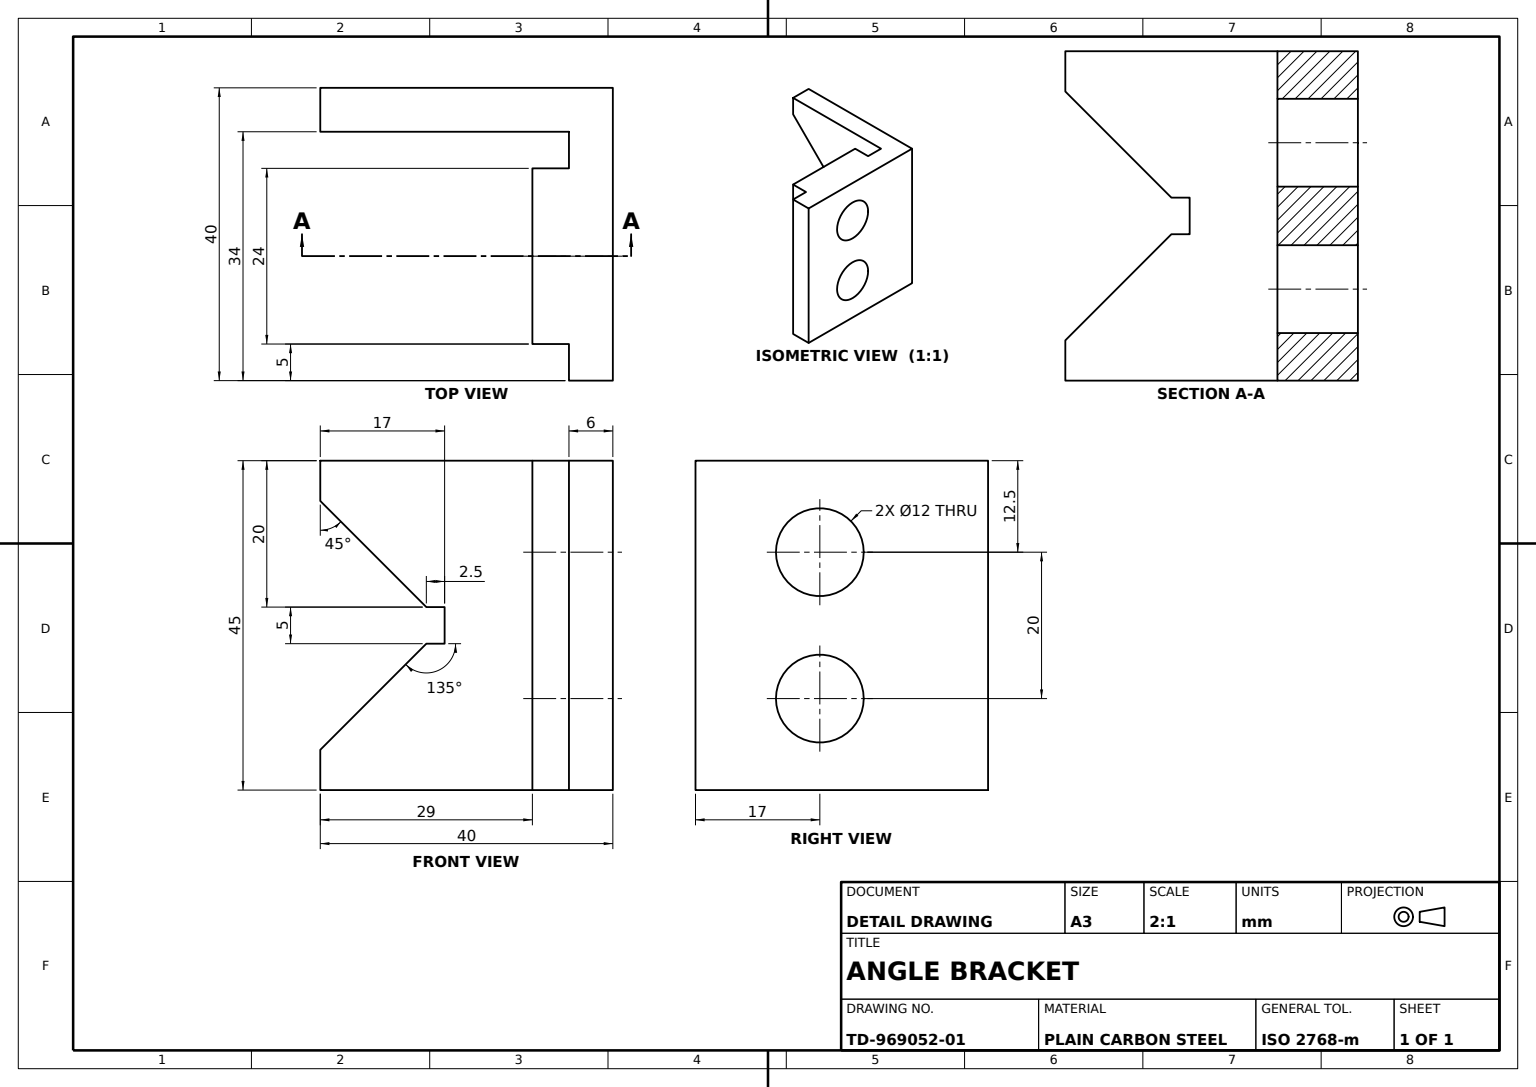
from build123d import *

# Parameters (mm, degrees)
BASE_PLATE_SKETCH_W        = 40
BASE_PLATE_SKETCH_H        = 45
BASE_PLATE_DEPTH           = 6
UPRIGHT_FLANGE_SKETCH_W    = 34
UPRIGHT_FLANGE_SKETCH_H    = 45
UPRIGHT_FLANGE_DEPTH       = 6
SUPPORT_WEB_SKETCH_W       = 5
SUPPORT_WEB_SKETCH_H       = 24
SUPPORT_WEB_DEPTH          = 45
CORNER_RELIEF_GROOVE_DEPTH = 45
MOUNTING_HOLES_SKETCH_R    = 6
MOUNTING_HOLES_2X_DEPTH    = 45


with BuildPart() as part:
    # Base Plate Sketch → Base Plate (new body)
    with BuildSketch(Plane.XY):
        with Locations((20, 22.5)):
            Rectangle(BASE_PLATE_SKETCH_W, BASE_PLATE_SKETCH_H)
    extrude(amount=BASE_PLATE_DEPTH)

    # Upright Flange Sketch → Upright Flange (add)
    with BuildSketch(Plane(origin=(40, 0, 0), x_dir=(0, 0, -1), z_dir=(1, 0, 0))):
        with Locations((-23, 22.5)):
            Rectangle(UPRIGHT_FLANGE_SKETCH_W, UPRIGHT_FLANGE_SKETCH_H)
    extrude(amount=-UPRIGHT_FLANGE_DEPTH)

    # Support Web Sketch → Support Web (add)
    with BuildSketch(Plane.XZ):
        with Locations((31.5, 23)):
            Rectangle(SUPPORT_WEB_SKETCH_W, SUPPORT_WEB_SKETCH_H)
    extrude(amount=-SUPPORT_WEB_DEPTH)

    # Corner Relief Groove Sketch → Corner Relief Groove (cut)
    with BuildSketch(Plane.XY.offset(6)):
        Polygon((0, 39.5), (0, 22.5), (17, 22.5), (17, 25), (14.5, 25), align=None)
        Polygon((17, 22.5), (0, 22.5), (0, 5.5), (14.5, 20), (17, 20), align=None)
    extrude(amount=-CORNER_RELIEF_GROOVE_DEPTH, mode=Mode.SUBTRACT)

    # Mounting Holes Sketch → Mounting Holes 2x (cut)
    with BuildSketch(Plane.ZY.offset(-29)):
        with Locations((23, 32.5)):
            Circle(MOUNTING_HOLES_SKETCH_R)
        with Locations((23, 12.5)):
            Circle(MOUNTING_HOLES_SKETCH_R)
    extrude(amount=-MOUNTING_HOLES_2X_DEPTH, mode=Mode.SUBTRACT)


solid = part.part
